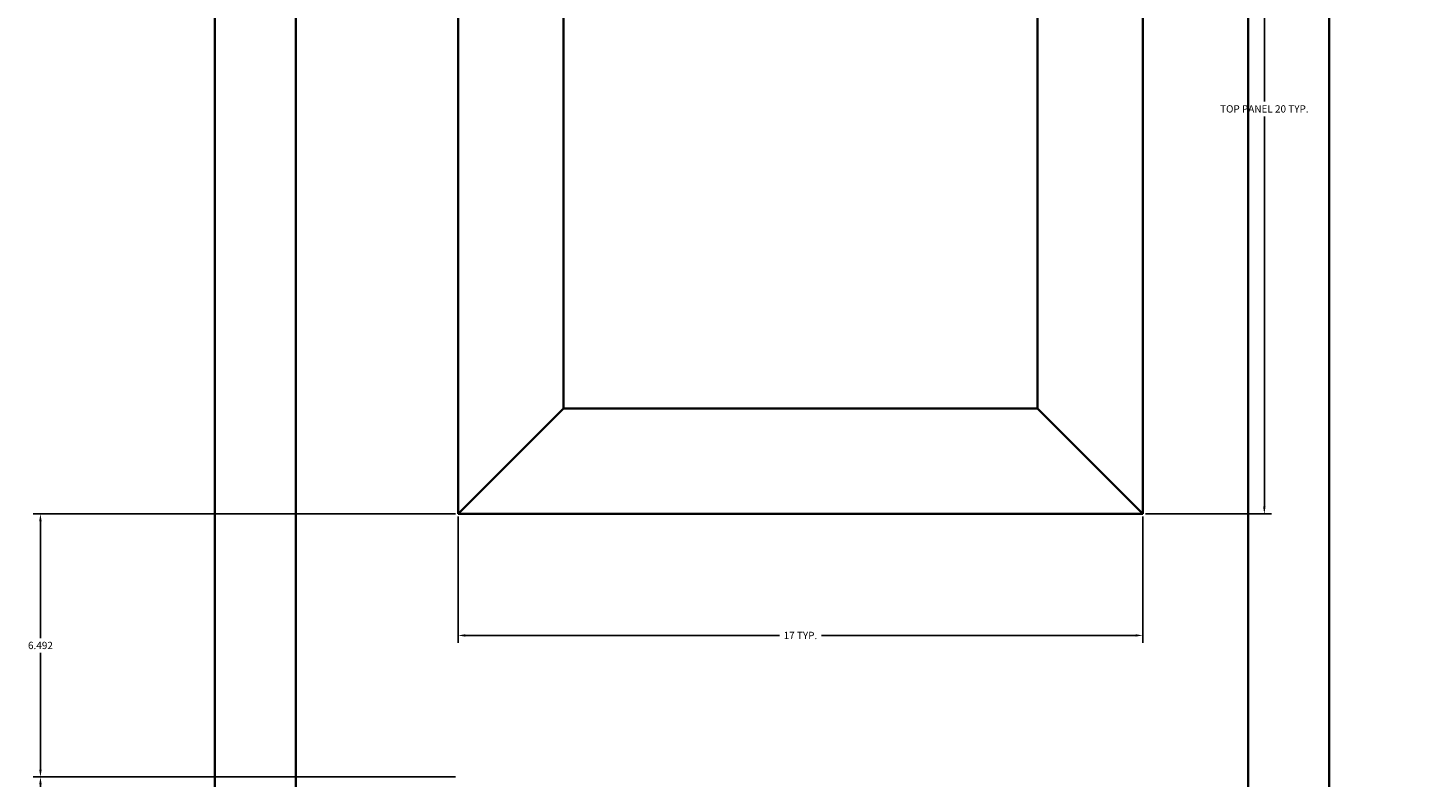
# Model space of a CAD drawing. Units: inches. Extents: x 3137 to 3299, y 1994 to 2089.
# Tile 12 of 14: x 3230 to 3264, y 2052 to 2070. Entities that reach past the tile are written whole.
import ezdxf

# ---------------------------------------------------------------- set-up
doc = ezdxf.new("R2010")
doc.units = ezdxf.units.IN
doc.header["$MEASUREMENT"] = 0
doc.layers.add('A-ANNO-DIMS', color=2, linetype='Continuous', lineweight=18)
doc.layers.add('A-DOOR', color=4, linetype='Continuous', lineweight=35)
doc.styles.get("Standard").update_dxf_attribs({"font": 'arial.ttf'})
doc.dimstyles.get("Standard").update_dxf_attribs({"dimtxt": 0.18, "dimasz": 0.18, "dimexe": 0.18, "dimexo": 0.0625, "dimgap": 0.09, "dimtad": 0, "dimtih": 1, "dimtoh": 1, "dimdec": 4, "dimzin": 0, "dimdsep": 46, "dimtxsty": 'Standard', "dimcen": 0.09, "dimadec": 0, "dimazin": 0, "dimtfac": 1, "dimtdec": 4, "dimtofl": 0, "dimtmove": 0, "dimatfit": 3, "dimfxl": 1, "dimtolj": 1, "dimtzin": 0, "dimarcsym": 0})

# ---------------------------------------------------------------- blocks, each defined once
blk = doc.blocks.new('DOOR-PANEL-RAISED-TOP')
for p, q in [((0, 19.99), (2.6, 17.39)), ((14.3, 17.39), (16.9, 19.99)), ((16.9, 0), (16.9, 19.99)), ((14.3, 2.6), (14.3, 17.39)), ((2.6, 2.6), (0, 0)), ((2.6, 2.6), (14.3, 2.6)), ((14.3, 2.6), (16.9, 0)), ((0, 0), (16.9, 0))]:
    blk.add_line(p, q)
for points in [[(0, 0), (0, 19.99), (16.9, 19.99)], [(2.6, 2.6), (2.6, 17.39), (14.3, 17.39)]]:
    blk.add_lwpolyline(points)
blk = doc.blocks.new('*D7')
at = {"layer": 'A-ANNO-DIMS', "color": 0, "lineweight": -2, "transparency": 16777216}
for p, q in [((3257.466, 2078.176), (3260.582, 2078.176)), ((3260.402, 2077.996), (3260.402, 2068.364)), ((3260.402, 2058.366), (3260.402, 2067.997)), ((3257.466, 2058.186), (3260.582, 2058.186))]:
    blk.add_line(p, q, dxfattribs=at)
at = {"layer": 'A-ANNO-DIMS', "color": 0, "transparency": 16777216}
for points in [[(3260.372, 2077.996), (3260.432, 2077.996), (3260.402, 2078.176)], [(3260.372, 2058.366), (3260.432, 2058.366), (3260.402, 2058.186)]]:
    blk.add_solid(points, dxfattribs=at)
at = {"layer": 'Defpoints', "color": 0, "transparency": 16777216}
for p in [(3257.404, 2078.176), (3260.402, 2078.176), (3257.404, 2058.186)]:
    blk.add_point(p, dxfattribs=at)
at = {"layer": 'A-ANNO-DIMS', "color": 0, "transparency": 16777216, "insert": (3260.402, 2068.181), "char_height": 0.18, "attachment_point": 5}
blk.add_mtext('\\A1;TOP PANEL 20 TYP.', dxfattribs=at)
blk = doc.blocks.new('*D8')
at = {"layer": 'A-ANNO-DIMS', "color": 0, "lineweight": -2, "transparency": 16777216}
for p, q in [((3240.504, 2058.123), (3240.504, 2055.007)), ((3257.404, 2058.123), (3257.404, 2055.007)), ((3240.684, 2055.187), (3248.434, 2055.187)), ((3257.224, 2055.187), (3249.474, 2055.187))]:
    blk.add_line(p, q, dxfattribs=at)
at = {"layer": 'A-ANNO-DIMS', "color": 0, "transparency": 16777216}
for points in [[(3240.684, 2055.217), (3240.684, 2055.157), (3240.504, 2055.187)], [(3257.224, 2055.217), (3257.224, 2055.157), (3257.404, 2055.187)]]:
    blk.add_solid(points, dxfattribs=at)
at = {"layer": 'Defpoints', "color": 0, "transparency": 16777216}
for p in [(3240.504, 2058.186), (3257.404, 2058.186), (3257.404, 2055.187)]:
    blk.add_point(p, dxfattribs=at)
at = {"layer": 'A-ANNO-DIMS', "color": 0, "transparency": 16777216, "insert": (3248.954, 2055.187), "char_height": 0.18, "attachment_point": 5}
blk.add_mtext('\\A1;17 TYP.', dxfattribs=at)
blk = doc.blocks.new('*D69')
at = {"layer": 'A-ANNO-DIMS', "color": 0, "lineweight": -2, "transparency": 16777216}
for p, q in [((3240.441, 2051.694), (3230.019, 2051.694)), ((3230.199, 2051.514), (3230.199, 2040.367)), ((3230.199, 2028.856), (3230.199, 2040.003)), ((3240.441, 2028.676), (3230.019, 2028.676))]:
    blk.add_line(p, q, dxfattribs=at)
at = {"layer": 'A-ANNO-DIMS', "color": 0, "transparency": 16777216}
for points in [[(3230.169, 2051.514), (3230.229, 2051.514), (3230.199, 2051.694)], [(3230.169, 2028.856), (3230.229, 2028.856), (3230.199, 2028.676)]]:
    blk.add_solid(points, dxfattribs=at)
at = {"layer": 'Defpoints', "color": 0, "transparency": 16777216}
for p in [(3230.199, 2051.694), (3240.504, 2051.694), (3240.504, 2028.676)]:
    blk.add_point(p, dxfattribs=at)
at = {"layer": 'A-ANNO-DIMS', "color": 0, "transparency": 16777216, "insert": (3230.199, 2040.185), "char_height": 0.18, "attachment_point": 5}
blk.add_mtext('\\A1;23.02', dxfattribs=at)
blk = doc.blocks.new('*D70')
at = {"layer": 'A-ANNO-DIMS', "color": 0, "lineweight": -2, "transparency": 16777216}
for p, q in [((3240.441, 2058.186), (3230.019, 2058.186)), ((3230.199, 2058.006), (3230.199, 2055.121)), ((3230.199, 2051.874), (3230.199, 2054.758)), ((3240.441, 2051.694), (3230.019, 2051.694))]:
    blk.add_line(p, q, dxfattribs=at)
at = {"layer": 'A-ANNO-DIMS', "color": 0, "transparency": 16777216}
for points in [[(3230.169, 2058.006), (3230.229, 2058.006), (3230.199, 2058.186)], [(3230.169, 2051.874), (3230.229, 2051.874), (3230.199, 2051.694)]]:
    blk.add_solid(points, dxfattribs=at)
at = {"layer": 'Defpoints', "color": 0, "transparency": 16777216}
for p in [(3230.199, 2058.186), (3240.504, 2058.186), (3240.504, 2051.694)]:
    blk.add_point(p, dxfattribs=at)
at = {"layer": 'A-ANNO-DIMS', "color": 0, "transparency": 16777216, "insert": (3230.199, 2054.94), "char_height": 0.18, "attachment_point": 5}
blk.add_mtext('\\A1;6.492', dxfattribs=at)

msp = doc.modelspace()

# ---------------------------------------------------------------- linework, layer by layer
at = {"layer": 'A-DOOR'}
for p, q in [((3260.0039, 2028.6759), (3260.0039, 2082.1756)), ((3262.0039, 2028.6759), (3262.0039, 2082.1756))]:
    msp.add_line(p, q, dxfattribs=at)
for points in [[(3234.5039, 2084.1756), (3294.5039, 2084.1756), (3294.5039, 2000.1756), (3234.5039, 2000.1756)], [(3236.5039, 2082.1756), (3292.5039, 2082.1756), (3292.5039, 2002.1756), (3236.5039, 2002.1756)]]:
    msp.add_lwpolyline(points, close=True, dxfattribs=at)

# ---------------------------------------------------------------- block references
msp.add_blockref('DOOR-PANEL-RAISED-TOP', (3240.504, 2058.186), dxfattribs=at)

# ---------------------------------------------------------------- dimensions: what is measured, and where the dimension line sits
at = {"layer": 'A-ANNO-DIMS'}
dim = msp.add_linear_dim(base=(3260.4024, 2078.1756), p1=(3257.4039, 2058.1855), p2=(3257.4039, 2078.1756), angle=90, text='TOP PANEL <> TYP.', dimstyle='Standard', override={"dimdec": 0, "dimrnd": 0, "dimzin": 0, "dimlunit": 2}, dxfattribs=at)
dim.commit()
dim.dimension.update_dxf_attribs({"geometry": '*D7', "text_midpoint": (3260.4024, 2068.1806)})
for base, p1, p2, override, picture, middle in [((3230.1989, 2058.1855), (3240.5039, 2051.6936), (3240.5039, 2058.1855), {"dimdec": 3, "dimlfac": 1, "dimrnd": 0, "dimzin": 0, "dimdsep": 46, "dimlunit": 2}, '*D70', (3230.1989, 2054.9395)), ((3230.1989, 2051.6936), (3240.5039, 2028.6759), (3240.5039, 2051.6936), {"dimdec": 2, "dimlfac": 1, "dimrnd": 0, "dimzin": 0, "dimdsep": 46, "dimlunit": 2}, '*D69', (3230.1989, 2040.1847))]:
    dim = msp.add_linear_dim(base=base, p1=p1, p2=p2, angle=90, dimstyle='Standard', override=override, dxfattribs=at)
    dim.commit()
    dim.dimension.update_dxf_attribs({"geometry": picture, "text_midpoint": middle})
dim = msp.add_linear_dim(base=(3257.4039, 2055.187), p1=(3240.5039, 2058.1855), p2=(3257.4039, 2058.1855), text='<> TYP.', dimstyle='Standard', override={"dimdec": 0, "dimrnd": 0, "dimzin": 0, "dimlunit": 2}, dxfattribs=at)
dim.commit()
dim.dimension.update_dxf_attribs({"geometry": '*D8', "text_midpoint": (3248.9539, 2055.187)})

doc.saveas('drawing.dxf')
